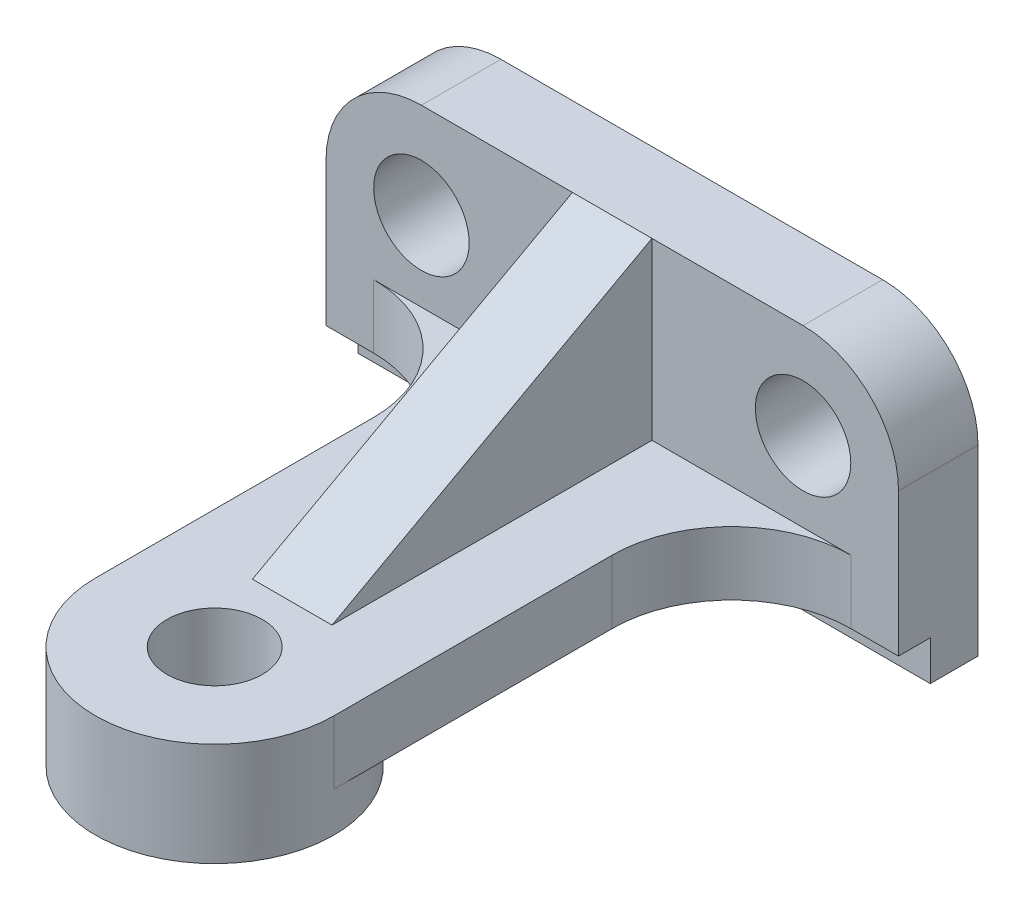
ISO-10303-21;
HEADER;
FILE_DESCRIPTION(('STEP AP214'),'2;1');
FILE_NAME('part.step','',(''),(''),'','','');
FILE_SCHEMA(('AUTOMOTIVE_DESIGN { 1 0 10303 214 1 1 1 1 }'));
ENDSEC;
DATA;
#1=APPLICATION_CONTEXT('core data for automotive mechanical design processes');
#2=APPLICATION_PROTOCOL_DEFINITION('international standard','automotive_design',2000,#1);
#3=PRODUCT_CONTEXT('',#1,'mechanical');
#4=PRODUCT('Part','Part','',(#3));
#5=PRODUCT_RELATED_PRODUCT_CATEGORY('part','',(#4));
#6=PRODUCT_DEFINITION_FORMATION('','',#4);
#7=PRODUCT_DEFINITION_CONTEXT('part definition',#1,'design');
#8=PRODUCT_DEFINITION('design','',#6,#7);
#9=PRODUCT_DEFINITION_SHAPE('','',#8);
#10=(LENGTH_UNIT() NAMED_UNIT(*) SI_UNIT(.MILLI.,.METRE.));
#11=(NAMED_UNIT(*) PLANE_ANGLE_UNIT() SI_UNIT($,.RADIAN.));
#12=(NAMED_UNIT(*) SI_UNIT($,.STERADIAN.) SOLID_ANGLE_UNIT());
#13=UNCERTAINTY_MEASURE_WITH_UNIT(LENGTH_MEASURE(1.E-05),#10,'distance_accuracy_value','');
#14=(GEOMETRIC_REPRESENTATION_CONTEXT(3) GLOBAL_UNCERTAINTY_ASSIGNED_CONTEXT((#13)) GLOBAL_UNIT_ASSIGNED_CONTEXT((#10,
#11,#12)) REPRESENTATION_CONTEXT('',''));
#15=CARTESIAN_POINT('',(0.,0.,0.));
#16=DIRECTION('',(0.,0.,1.));
#17=DIRECTION('',(1.,0.,0.));
#18=AXIS2_PLACEMENT_3D('',#15,#16,#17);
#19=CARTESIAN_POINT('',(42.,-9.99999999999999,50.2459304214752));
#20=DIRECTION('',(0.,0.877458255915555,0.479653009086393));
#21=DIRECTION('',(0.,-0.479653009086394,0.877458255915555));
#22=AXIS2_PLACEMENT_3D('',#19,#20,#21);
#23=PLANE('',#22);
#24=DIRECTION('',(0.,-0.479653009086393,0.877458255915555));
#25=VECTOR('',#24,1.);
#26=CARTESIAN_POINT('',(41.,12.,10.));
#27=LINE('',#26,#25);
#28=CARTESIAN_POINT('',(41.,12.,10.));
#29=VERTEX_POINT('',#28);
#30=CARTESIAN_POINT('',(41.,-9.99999999999999,50.2459304214752));
#31=VERTEX_POINT('',#30);
#32=EDGE_CURVE('E177',#29,#31,#27,.T.);
#33=ORIENTED_EDGE('',*,*,#32,.F.);
#34=DIRECTION('',(-1.,0.,0.));
#35=VECTOR('',#34,1.);
#36=CARTESIAN_POINT('',(42.,12.,10.));
#37=LINE('',#36,#35);
#38=CARTESIAN_POINT('',(31.,12.,10.));
#39=VERTEX_POINT('',#38);
#40=EDGE_CURVE('E186',#29,#39,#37,.T.);
#41=ORIENTED_EDGE('',*,*,#40,.T.);
#42=DIRECTION('',(0.,0.479653009086393,-0.877458255915555));
#43=VECTOR('',#42,1.);
#44=CARTESIAN_POINT('',(31.,-9.99999999999999,50.2459304214752));
#45=LINE('',#44,#43);
#46=CARTESIAN_POINT('',(31.,-9.99999999999999,50.2459304214752));
#47=VERTEX_POINT('',#46);
#48=EDGE_CURVE('E189',#47,#39,#45,.T.);
#49=ORIENTED_EDGE('',*,*,#48,.F.);
#50=DIRECTION('',(-1.,0.,0.));
#51=VECTOR('',#50,1.);
#52=CARTESIAN_POINT('',(42.,-9.99999999999999,50.2459304214752));
#53=LINE('',#52,#51);
#54=EDGE_CURVE('E171',#31,#47,#53,.T.);
#55=ORIENTED_EDGE('',*,*,#54,.F.);
#56=EDGE_LOOP('',(#33,#41,#49,#55));
#57=FACE_BOUND('',#56,.T.);
#58=ADVANCED_FACE('F44',(#57),#23,.T.);
#59=CARTESIAN_POINT('',(12.,0.,10.));
#60=DIRECTION('',(0.,0.,1.));
#61=DIRECTION('',(1.,0.,0.));
#62=AXIS2_PLACEMENT_3D('',#59,#60,#61);
#63=PLANE('',#62);
#64=CARTESIAN_POINT('',(60.,0.,10.));
#65=DIRECTION('',(0.,0.,1.));
#66=DIRECTION('',(1.,0.,0.));
#67=AXIS2_PLACEMENT_3D('',#64,#65,#66);
#68=CIRCLE('',#67,6.);
#69=CARTESIAN_POINT('',(66.,0.,10.));
#70=VERTEX_POINT('',#69);
#71=EDGE_CURVE('E205',#70,#70,#68,.T.);
#72=ORIENTED_EDGE('',*,*,#71,.F.);
#73=EDGE_LOOP('',(#72));
#74=FACE_BOUND('',#73,.T.);
#75=DIRECTION('',(-1.,0.,0.));
#76=VECTOR('',#75,1.);
#77=CARTESIAN_POINT('',(12.,12.,10.));
#78=LINE('',#77,#76);
#79=CARTESIAN_POINT('',(60.,12.,10.));
#80=VERTEX_POINT('',#79);
#81=EDGE_CURVE('E285',#80,#29,#78,.T.);
#82=ORIENTED_EDGE('',*,*,#81,.T.);
#83=DIRECTION('',(0.,1.,0.));
#84=VECTOR('',#83,1.);
#85=CARTESIAN_POINT('',(41.,-9.99999999999999,10.));
#86=LINE('',#85,#84);
#87=CARTESIAN_POINT('',(41.,-9.99999999999999,10.));
#88=VERTEX_POINT('',#87);
#89=EDGE_CURVE('E178',#88,#29,#86,.T.);
#90=ORIENTED_EDGE('',*,*,#89,.F.);
#91=DIRECTION('',(1.,0.,0.));
#92=VECTOR('',#91,1.);
#93=CARTESIAN_POINT('',(5.99999999999989,-9.99999999999999,10.));
#94=LINE('',#93,#92);
#95=CARTESIAN_POINT('',(66.0000000000001,-9.99999999999999,10.));
#96=VERTEX_POINT('',#95);
#97=EDGE_CURVE('E172',#88,#96,#94,.T.);
#98=ORIENTED_EDGE('',*,*,#97,.T.);
#99=DIRECTION('',(0.,-1.,0.));
#100=VECTOR('',#99,1.);
#101=CARTESIAN_POINT('',(66.0000000000001,-9.99999999999999,10.));
#102=LINE('',#101,#100);
#103=CARTESIAN_POINT('',(66.0000000000001,-18.,10.));
#104=VERTEX_POINT('',#103);
#105=EDGE_CURVE('E248',#96,#104,#102,.T.);
#106=ORIENTED_EDGE('',*,*,#105,.T.);
#107=DIRECTION('',(-1.,0.,0.));
#108=VECTOR('',#107,1.);
#109=CARTESIAN_POINT('',(72.,-18.,10.));
#110=LINE('',#109,#108);
#111=CARTESIAN_POINT('',(72.,-18.,10.));
#112=VERTEX_POINT('',#111);
#113=EDGE_CURVE('E271',#112,#104,#110,.T.);
#114=ORIENTED_EDGE('',*,*,#113,.F.);
#115=DIRECTION('',(0.,1.,0.));
#116=VECTOR('',#115,1.);
#117=CARTESIAN_POINT('',(72.,-23.,10.));
#118=LINE('',#117,#116);
#119=CARTESIAN_POINT('',(72.,0.,10.));
#120=VERTEX_POINT('',#119);
#121=EDGE_CURVE('E281',#112,#120,#118,.T.);
#122=ORIENTED_EDGE('',*,*,#121,.T.);
#123=CARTESIAN_POINT('',(60.,0.,10.));
#124=DIRECTION('',(0.,0.,1.));
#125=DIRECTION('',(1.,0.,0.));
#126=AXIS2_PLACEMENT_3D('',#123,#124,#125);
#127=CIRCLE('',#126,12.);
#128=EDGE_CURVE('E284',#120,#80,#127,.T.);
#129=ORIENTED_EDGE('',*,*,#128,.T.);
#130=EDGE_LOOP('',(#82,#90,#98,#106,#114,#122,#129));
#131=FACE_BOUND('',#130,.T.);
#132=ADVANCED_FACE('F332',(#74,#131),#63,.T.);
#133=CARTESIAN_POINT('',(72.,-18.,6.));
#134=DIRECTION('',(0.,1.,0.));
#135=DIRECTION('',(0.,0.,1.));
#136=AXIS2_PLACEMENT_3D('',#133,#134,#135);
#137=PLANE('',#136);
#138=CARTESIAN_POINT('',(36.,-18.,60.));
#139=DIRECTION('',(0.,-1.,0.));
#140=DIRECTION('',(0.,0.,-1.));
#141=AXIS2_PLACEMENT_3D('',#138,#139,#140);
#142=CIRCLE('',#141,15.);
#143=CARTESIAN_POINT('',(21.,-18.,60.));
#144=VERTEX_POINT('',#143);
#145=CARTESIAN_POINT('',(51.,-18.,60.));
#146=VERTEX_POINT('',#145);
#147=EDGE_CURVE('E206',#144,#146,#142,.T.);
#148=ORIENTED_EDGE('',*,*,#147,.F.);
#149=DIRECTION('',(0.,0.,-1.));
#150=VECTOR('',#149,1.);
#151=CARTESIAN_POINT('',(21.,-18.,60.));
#152=LINE('',#151,#150);
#153=CARTESIAN_POINT('',(21.,-18.,25.0000000000001));
#154=VERTEX_POINT('',#153);
#155=EDGE_CURVE('E217',#144,#154,#152,.T.);
#156=ORIENTED_EDGE('',*,*,#155,.T.);
#157=CARTESIAN_POINT('',(6.,-18.,25.));
#158=DIRECTION('',(0.,1.,0.));
#159=DIRECTION('',(0.,0.,1.));
#160=AXIS2_PLACEMENT_3D('',#157,#158,#159);
#161=CIRCLE('',#160,15.);
#162=CARTESIAN_POINT('',(6.,-18.,10.));
#163=VERTEX_POINT('',#162);
#164=EDGE_CURVE('E58',#154,#163,#161,.T.);
#165=ORIENTED_EDGE('',*,*,#164,.T.);
#166=CARTESIAN_POINT('',(0.,-18.,10.));
#167=VERTEX_POINT('',#166);
#168=EDGE_CURVE('E264',#163,#167,#110,.T.);
#169=ORIENTED_EDGE('',*,*,#168,.T.);
#170=DIRECTION('',(0.,0.,-1.));
#171=VECTOR('',#170,1.);
#172=CARTESIAN_POINT('',(0.,-18.,6.));
#173=LINE('',#172,#171);
#174=CARTESIAN_POINT('',(0.,-18.,6.));
#175=VERTEX_POINT('',#174);
#176=EDGE_CURVE('E246',#167,#175,#173,.T.);
#177=ORIENTED_EDGE('',*,*,#176,.T.);
#178=DIRECTION('',(-1.,0.,0.));
#179=VECTOR('',#178,1.);
#180=CARTESIAN_POINT('',(72.,-18.,6.));
#181=LINE('',#180,#179);
#182=CARTESIAN_POINT('',(72.,-18.,6.));
#183=VERTEX_POINT('',#182);
#184=EDGE_CURVE('E272',#183,#175,#181,.T.);
#185=ORIENTED_EDGE('',*,*,#184,.F.);
#186=DIRECTION('',(0.,0.,-1.));
#187=VECTOR('',#186,1.);
#188=CARTESIAN_POINT('',(72.,-18.,6.));
#189=LINE('',#188,#187);
#190=EDGE_CURVE('E67',#112,#183,#189,.T.);
#191=ORIENTED_EDGE('',*,*,#190,.F.);
#192=ORIENTED_EDGE('',*,*,#113,.T.);
#193=CARTESIAN_POINT('',(66.,-18.,25.));
#194=DIRECTION('',(0.,1.,0.));
#195=DIRECTION('',(0.,0.,-1.));
#196=AXIS2_PLACEMENT_3D('',#193,#194,#195);
#197=CIRCLE('',#196,15.);
#198=CARTESIAN_POINT('',(51.,-18.,25.0000000000001));
#199=VERTEX_POINT('',#198);
#200=EDGE_CURVE('E237',#104,#199,#197,.T.);
#201=ORIENTED_EDGE('',*,*,#200,.T.);
#202=DIRECTION('',(0.,0.,1.));
#203=VECTOR('',#202,1.);
#204=CARTESIAN_POINT('',(51.,-18.,60.));
#205=LINE('',#204,#203);
#206=EDGE_CURVE('E224',#199,#146,#205,.T.);
#207=ORIENTED_EDGE('',*,*,#206,.T.);
#208=EDGE_LOOP('',(#148,#156,#165,#169,#177,#185,#191,#192,#201,#207));
#209=FACE_BOUND('',#208,.T.);
#210=ADVANCED_FACE('F344',(#209),#137,.F.);
#211=CARTESIAN_POINT('',(12.,0.,10.));
#212=DIRECTION('',(0.,0.,-1.));
#213=DIRECTION('',(-1.,0.,0.));
#214=AXIS2_PLACEMENT_3D('',#211,#212,#213);
#215=CYLINDRICAL_SURFACE('',#214,12.);
#216=CARTESIAN_POINT('',(12.,0.,0.));
#217=DIRECTION('',(0.,0.,1.));
#218=DIRECTION('',(1.,0.,0.));
#219=AXIS2_PLACEMENT_3D('',#216,#217,#218);
#220=CIRCLE('',#219,12.);
#221=CARTESIAN_POINT('',(12.,12.,0.));
#222=VERTEX_POINT('',#221);
#223=CARTESIAN_POINT('',(0.,0.,0.));
#224=VERTEX_POINT('',#223);
#225=EDGE_CURVE('E267',#222,#224,#220,.T.);
#226=ORIENTED_EDGE('',*,*,#225,.T.);
#227=DIRECTION('',(0.,0.,-1.));
#228=VECTOR('',#227,1.);
#229=CARTESIAN_POINT('',(0.,0.,10.));
#230=LINE('',#229,#228);
#231=CARTESIAN_POINT('',(0.,0.,10.));
#232=VERTEX_POINT('',#231);
#233=EDGE_CURVE('E11',#232,#224,#230,.T.);
#234=ORIENTED_EDGE('',*,*,#233,.F.);
#235=CARTESIAN_POINT('',(12.,0.,10.));
#236=DIRECTION('',(0.,0.,1.));
#237=DIRECTION('',(1.,0.,0.));
#238=AXIS2_PLACEMENT_3D('',#235,#236,#237);
#239=CIRCLE('',#238,12.);
#240=CARTESIAN_POINT('',(12.,12.,10.));
#241=VERTEX_POINT('',#240);
#242=EDGE_CURVE('E273',#241,#232,#239,.T.);
#243=ORIENTED_EDGE('',*,*,#242,.F.);
#244=DIRECTION('',(0.,0.,-1.));
#245=VECTOR('',#244,1.);
#246=CARTESIAN_POINT('',(12.,12.,10.));
#247=LINE('',#246,#245);
#248=EDGE_CURVE('E290',#241,#222,#247,.T.);
#249=ORIENTED_EDGE('',*,*,#248,.T.);
#250=EDGE_LOOP('',(#226,#234,#243,#249));
#251=FACE_BOUND('',#250,.T.);
#252=ADVANCED_FACE('F50',(#251),#215,.T.);
#253=CARTESIAN_POINT('',(0.,0.,10.));
#254=DIRECTION('',(1.,0.,0.));
#255=DIRECTION('',(0.,0.,-1.));
#256=AXIS2_PLACEMENT_3D('',#253,#254,#255);
#257=PLANE('',#256);
#258=DIRECTION('',(0.,-1.,0.));
#259=VECTOR('',#258,1.);
#260=CARTESIAN_POINT('',(0.,0.,10.));
#261=LINE('',#260,#259);
#262=EDGE_CURVE('E280',#232,#167,#261,.T.);
#263=ORIENTED_EDGE('',*,*,#262,.F.);
#264=ORIENTED_EDGE('',*,*,#233,.T.);
#265=DIRECTION('',(0.,-1.,0.));
#266=VECTOR('',#265,1.);
#267=CARTESIAN_POINT('',(0.,0.,0.));
#268=LINE('',#267,#266);
#269=CARTESIAN_POINT('',(0.,-23.,0.));
#270=VERTEX_POINT('',#269);
#271=EDGE_CURVE('E287',#224,#270,#268,.T.);
#272=ORIENTED_EDGE('',*,*,#271,.T.);
#273=DIRECTION('',(0.,0.,-1.));
#274=VECTOR('',#273,1.);
#275=CARTESIAN_POINT('',(0.,-23.,10.));
#276=LINE('',#275,#274);
#277=CARTESIAN_POINT('',(0.,-23.,6.));
#278=VERTEX_POINT('',#277);
#279=EDGE_CURVE('E52',#278,#270,#276,.T.);
#280=ORIENTED_EDGE('',*,*,#279,.F.);
#281=DIRECTION('',(0.,-1.,0.));
#282=VECTOR('',#281,1.);
#283=CARTESIAN_POINT('',(0.,-23.,6.));
#284=LINE('',#283,#282);
#285=EDGE_CURVE('E257',#175,#278,#284,.T.);
#286=ORIENTED_EDGE('',*,*,#285,.F.);
#287=ORIENTED_EDGE('',*,*,#176,.F.);
#288=EDGE_LOOP('',(#263,#264,#272,#280,#286,#287));
#289=FACE_BOUND('',#288,.T.);
#290=ADVANCED_FACE('F319',(#289),#257,.F.);
#291=CARTESIAN_POINT('',(0.,-23.,10.));
#292=DIRECTION('',(0.,1.,0.));
#293=DIRECTION('',(0.,0.,1.));
#294=AXIS2_PLACEMENT_3D('',#291,#292,#293);
#295=PLANE('',#294);
#296=DIRECTION('',(0.,0.,-1.));
#297=VECTOR('',#296,1.);
#298=CARTESIAN_POINT('',(72.,-23.,10.));
#299=LINE('',#298,#297);
#300=CARTESIAN_POINT('',(72.,-23.,6.));
#301=VERTEX_POINT('',#300);
#302=CARTESIAN_POINT('',(72.,-23.,0.));
#303=VERTEX_POINT('',#302);
#304=EDGE_CURVE('E307',#301,#303,#299,.T.);
#305=ORIENTED_EDGE('',*,*,#304,.F.);
#306=DIRECTION('',(-1.,0.,0.));
#307=VECTOR('',#306,1.);
#308=CARTESIAN_POINT('',(72.,-23.,6.));
#309=LINE('',#308,#307);
#310=EDGE_CURVE('E270',#301,#278,#309,.T.);
#311=ORIENTED_EDGE('',*,*,#310,.T.);
#312=ORIENTED_EDGE('',*,*,#279,.T.);
#313=DIRECTION('',(1.,0.,0.));
#314=VECTOR('',#313,1.);
#315=CARTESIAN_POINT('',(0.,-23.,0.));
#316=LINE('',#315,#314);
#317=EDGE_CURVE('E291',#270,#303,#316,.T.);
#318=ORIENTED_EDGE('',*,*,#317,.T.);
#319=EDGE_LOOP('',(#305,#311,#312,#318));
#320=FACE_BOUND('',#319,.T.);
#321=ADVANCED_FACE('F312',(#320),#295,.F.);
#322=CARTESIAN_POINT('',(72.,-23.,10.));
#323=DIRECTION('',(-1.,0.,0.));
#324=DIRECTION('',(0.,0.,1.));
#325=AXIS2_PLACEMENT_3D('',#322,#323,#324);
#326=PLANE('',#325);
#327=ORIENTED_EDGE('',*,*,#190,.T.);
#328=DIRECTION('',(0.,-1.,0.));
#329=VECTOR('',#328,1.);
#330=CARTESIAN_POINT('',(72.,-23.,6.));
#331=LINE('',#330,#329);
#332=EDGE_CURVE('E258',#183,#301,#331,.T.);
#333=ORIENTED_EDGE('',*,*,#332,.T.);
#334=ORIENTED_EDGE('',*,*,#304,.T.);
#335=DIRECTION('',(0.,1.,0.));
#336=VECTOR('',#335,1.);
#337=CARTESIAN_POINT('',(72.,-23.,0.));
#338=LINE('',#337,#336);
#339=CARTESIAN_POINT('',(72.,0.,0.));
#340=VERTEX_POINT('',#339);
#341=EDGE_CURVE('E298',#303,#340,#338,.T.);
#342=ORIENTED_EDGE('',*,*,#341,.T.);
#343=DIRECTION('',(0.,0.,-1.));
#344=VECTOR('',#343,1.);
#345=CARTESIAN_POINT('',(72.,0.,10.));
#346=LINE('',#345,#344);
#347=EDGE_CURVE('E306',#120,#340,#346,.T.);
#348=ORIENTED_EDGE('',*,*,#347,.F.);
#349=ORIENTED_EDGE('',*,*,#121,.F.);
#350=EDGE_LOOP('',(#327,#333,#334,#342,#348,#349));
#351=FACE_BOUND('',#350,.T.);
#352=ADVANCED_FACE('F327',(#351),#326,.F.);
#353=CARTESIAN_POINT('',(60.,0.,10.));
#354=DIRECTION('',(0.,0.,-1.));
#355=DIRECTION('',(-1.,0.,0.));
#356=AXIS2_PLACEMENT_3D('',#353,#354,#355);
#357=CYLINDRICAL_SURFACE('',#356,12.);
#358=CARTESIAN_POINT('',(60.,0.,0.));
#359=DIRECTION('',(0.,0.,1.));
#360=DIRECTION('',(1.,0.,0.));
#361=AXIS2_PLACEMENT_3D('',#358,#359,#360);
#362=CIRCLE('',#361,12.);
#363=CARTESIAN_POINT('',(60.,12.,0.));
#364=VERTEX_POINT('',#363);
#365=EDGE_CURVE('E296',#340,#364,#362,.T.);
#366=ORIENTED_EDGE('',*,*,#365,.T.);
#367=DIRECTION('',(0.,0.,-1.));
#368=VECTOR('',#367,1.);
#369=CARTESIAN_POINT('',(60.,12.,10.));
#370=LINE('',#369,#368);
#371=EDGE_CURVE('E303',#80,#364,#370,.T.);
#372=ORIENTED_EDGE('',*,*,#371,.F.);
#373=ORIENTED_EDGE('',*,*,#128,.F.);
#374=ORIENTED_EDGE('',*,*,#347,.T.);
#375=EDGE_LOOP('',(#366,#372,#373,#374));
#376=FACE_BOUND('',#375,.T.);
#377=ADVANCED_FACE('F333',(#376),#357,.T.);
#378=CARTESIAN_POINT('',(12.,12.,10.));
#379=DIRECTION('',(0.,-1.,0.));
#380=DIRECTION('',(1.,0.,0.));
#381=AXIS2_PLACEMENT_3D('',#378,#379,#380);
#382=PLANE('',#381);
#383=DIRECTION('',(-1.,0.,0.));
#384=VECTOR('',#383,1.);
#385=CARTESIAN_POINT('',(12.,12.,0.));
#386=LINE('',#385,#384);
#387=EDGE_CURVE('E278',#364,#222,#386,.T.);
#388=ORIENTED_EDGE('',*,*,#387,.T.);
#389=ORIENTED_EDGE('',*,*,#248,.F.);
#390=DIRECTION('',(-1.,0.,0.));
#391=VECTOR('',#390,1.);
#392=CARTESIAN_POINT('',(30.,12.,10.));
#393=LINE('',#392,#391);
#394=EDGE_CURVE('E350',#39,#241,#393,.T.);
#395=ORIENTED_EDGE('',*,*,#394,.F.);
#396=ORIENTED_EDGE('',*,*,#40,.F.);
#397=ORIENTED_EDGE('',*,*,#81,.F.);
#398=ORIENTED_EDGE('',*,*,#371,.T.);
#399=EDGE_LOOP('',(#388,#389,#395,#396,#397,#398));
#400=FACE_BOUND('',#399,.T.);
#401=ADVANCED_FACE('F354',(#400),#382,.F.);
#402=DIRECTION('',(0.,-1.,0.));
#403=VECTOR('',#402,1.);
#404=CARTESIAN_POINT('',(5.9999999999999,-9.99999999999999,10.));
#405=LINE('',#404,#403);
#406=CARTESIAN_POINT('',(5.9999999999999,-9.99999999999999,10.));
#407=VERTEX_POINT('',#406);
#408=EDGE_CURVE('E255',#407,#163,#405,.T.);
#409=ORIENTED_EDGE('',*,*,#408,.F.);
#410=DIRECTION('',(-1.,0.,0.));
#411=VECTOR('',#410,1.);
#412=CARTESIAN_POINT('',(30.,-9.99999999999999,10.));
#413=LINE('',#412,#411);
#414=CARTESIAN_POINT('',(31.,-9.99999999999999,10.));
#415=VERTEX_POINT('',#414);
#416=EDGE_CURVE('E192',#415,#407,#413,.T.);
#417=ORIENTED_EDGE('',*,*,#416,.F.);
#418=DIRECTION('',(0.,-1.,0.));
#419=VECTOR('',#418,1.);
#420=CARTESIAN_POINT('',(31.,12.,10.));
#421=LINE('',#420,#419);
#422=EDGE_CURVE('E357',#39,#415,#421,.T.);
#423=ORIENTED_EDGE('',*,*,#422,.F.);
#424=ORIENTED_EDGE('',*,*,#394,.T.);
#425=ORIENTED_EDGE('',*,*,#242,.T.);
#426=ORIENTED_EDGE('',*,*,#262,.T.);
#427=ORIENTED_EDGE('',*,*,#168,.F.);
#428=EDGE_LOOP('',(#409,#417,#423,#424,#425,#426,#427));
#429=FACE_BOUND('',#428,.T.);
#430=CARTESIAN_POINT('',(12.,0.,10.));
#431=DIRECTION('',(0.,0.,-1.));
#432=DIRECTION('',(0.,1.,0.));
#433=AXIS2_PLACEMENT_3D('',#430,#431,#432);
#434=CIRCLE('',#433,6.);
#435=CARTESIAN_POINT('',(12.,6.,10.));
#436=VERTEX_POINT('',#435);
#437=EDGE_CURVE('E188',#436,#436,#434,.F.);
#438=ORIENTED_EDGE('',*,*,#437,.F.);
#439=EDGE_LOOP('',(#438));
#440=FACE_BOUND('',#439,.T.);
#441=ADVANCED_FACE('F342',(#429,#440),#63,.T.);
#442=CARTESIAN_POINT('',(12.,0.,0.));
#443=DIRECTION('',(0.,0.,1.));
#444=DIRECTION('',(1.,0.,0.));
#445=AXIS2_PLACEMENT_3D('',#442,#443,#444);
#446=PLANE('',#445);
#447=CARTESIAN_POINT('',(12.,0.,0.));
#448=DIRECTION('',(0.,0.,1.));
#449=DIRECTION('',(1.,0.,0.));
#450=AXIS2_PLACEMENT_3D('',#447,#448,#449);
#451=CIRCLE('',#450,6.);
#452=CARTESIAN_POINT('',(18.,0.,0.));
#453=VERTEX_POINT('',#452);
#454=EDGE_CURVE('E202',#453,#453,#451,.T.);
#455=ORIENTED_EDGE('',*,*,#454,.T.);
#456=EDGE_LOOP('',(#455));
#457=FACE_BOUND('',#456,.T.);
#458=CARTESIAN_POINT('',(60.,0.,0.));
#459=DIRECTION('',(0.,0.,1.));
#460=DIRECTION('',(1.,0.,0.));
#461=AXIS2_PLACEMENT_3D('',#458,#459,#460);
#462=CIRCLE('',#461,6.);
#463=CARTESIAN_POINT('',(66.,0.,0.));
#464=VERTEX_POINT('',#463);
#465=EDGE_CURVE('E209',#464,#464,#462,.T.);
#466=ORIENTED_EDGE('',*,*,#465,.T.);
#467=EDGE_LOOP('',(#466));
#468=FACE_BOUND('',#467,.T.);
#469=ORIENTED_EDGE('',*,*,#225,.F.);
#470=ORIENTED_EDGE('',*,*,#387,.F.);
#471=ORIENTED_EDGE('',*,*,#365,.F.);
#472=ORIENTED_EDGE('',*,*,#341,.F.);
#473=ORIENTED_EDGE('',*,*,#317,.F.);
#474=ORIENTED_EDGE('',*,*,#271,.F.);
#475=EDGE_LOOP('',(#469,#470,#471,#472,#473,#474));
#476=FACE_BOUND('',#475,.T.);
#477=ADVANCED_FACE('F321',(#457,#468,#476),#446,.F.);
#478=CARTESIAN_POINT('',(72.,-23.,6.));
#479=DIRECTION('',(0.,0.,-1.));
#480=DIRECTION('',(-1.,0.,0.));
#481=AXIS2_PLACEMENT_3D('',#478,#479,#480);
#482=PLANE('',#481);
#483=ORIENTED_EDGE('',*,*,#285,.T.);
#484=ORIENTED_EDGE('',*,*,#310,.F.);
#485=ORIENTED_EDGE('',*,*,#332,.F.);
#486=ORIENTED_EDGE('',*,*,#184,.T.);
#487=EDGE_LOOP('',(#483,#484,#485,#486));
#488=FACE_BOUND('',#487,.T.);
#489=ADVANCED_FACE('F336',(#488),#482,.F.);
#490=CARTESIAN_POINT('',(36.,-9.99999999999999,60.));
#491=DIRECTION('',(0.,-1.,0.));
#492=DIRECTION('',(0.,0.,-1.));
#493=AXIS2_PLACEMENT_3D('',#490,#491,#492);
#494=CYLINDRICAL_SURFACE('',#493,15.);
#495=DIRECTION('',(0.,-1.,0.));
#496=VECTOR('',#495,1.);
#497=CARTESIAN_POINT('',(21.,-9.99999999999999,60.));
#498=LINE('',#497,#496);
#499=CARTESIAN_POINT('',(21.,-9.99999999999999,60.));
#500=VERTEX_POINT('',#499);
#501=EDGE_CURVE('E236',#500,#144,#498,.T.);
#502=ORIENTED_EDGE('',*,*,#501,.T.);
#503=ORIENTED_EDGE('',*,*,#147,.T.);
#504=DIRECTION('',(0.,-1.,0.));
#505=VECTOR('',#504,1.);
#506=CARTESIAN_POINT('',(51.,-9.99999999999999,60.));
#507=LINE('',#506,#505);
#508=CARTESIAN_POINT('',(51.,-9.99999999999999,60.));
#509=VERTEX_POINT('',#508);
#510=EDGE_CURVE('E242',#509,#146,#507,.T.);
#511=ORIENTED_EDGE('',*,*,#510,.F.);
#512=CARTESIAN_POINT('',(36.,-9.99999999999999,60.));
#513=DIRECTION('',(0.,-1.,0.));
#514=DIRECTION('',(0.,0.,-1.));
#515=AXIS2_PLACEMENT_3D('',#512,#513,#514);
#516=CIRCLE('',#515,15.);
#517=EDGE_CURVE('E220',#509,#500,#516,.T.);
#518=ORIENTED_EDGE('',*,*,#517,.T.);
#519=EDGE_LOOP('',(#502,#503,#511,#518));
#520=FACE_BOUND('',#519,.T.);
#521=CARTESIAN_POINT('',(36.,-23.,60.));
#522=DIRECTION('',(0.,-1.,0.));
#523=DIRECTION('',(0.,0.,-1.));
#524=AXIS2_PLACEMENT_3D('',#521,#522,#523);
#525=CIRCLE('',#524,15.);
#526=CARTESIAN_POINT('',(36.,-23.,45.));
#527=VERTEX_POINT('',#526);
#528=EDGE_CURVE('E213',#527,#527,#525,.T.);
#529=ORIENTED_EDGE('',*,*,#528,.F.);
#530=EDGE_LOOP('',(#529));
#531=FACE_BOUND('',#530,.T.);
#532=ADVANCED_FACE('F374',(#520,#531),#494,.T.);
#533=CARTESIAN_POINT('',(51.,-9.99999999999999,60.));
#534=DIRECTION('',(1.,0.,0.));
#535=DIRECTION('',(0.,0.,-1.));
#536=AXIS2_PLACEMENT_3D('',#533,#534,#535);
#537=PLANE('',#536);
#538=ORIENTED_EDGE('',*,*,#206,.F.);
#539=DIRECTION('',(0.,-1.,0.));
#540=VECTOR('',#539,1.);
#541=CARTESIAN_POINT('',(51.,-9.99999999999999,25.0000000000001));
#542=LINE('',#541,#540);
#543=CARTESIAN_POINT('',(51.,-9.99999999999999,25.0000000000001));
#544=VERTEX_POINT('',#543);
#545=EDGE_CURVE('E250',#544,#199,#542,.T.);
#546=ORIENTED_EDGE('',*,*,#545,.F.);
#547=DIRECTION('',(0.,0.,1.));
#548=VECTOR('',#547,1.);
#549=CARTESIAN_POINT('',(51.,-9.99999999999999,60.));
#550=LINE('',#549,#548);
#551=EDGE_CURVE('E231',#544,#509,#550,.T.);
#552=ORIENTED_EDGE('',*,*,#551,.T.);
#553=ORIENTED_EDGE('',*,*,#510,.T.);
#554=EDGE_LOOP('',(#538,#546,#552,#553));
#555=FACE_BOUND('',#554,.T.);
#556=ADVANCED_FACE('F378',(#555),#537,.T.);
#557=CARTESIAN_POINT('',(66.,-9.99999999999999,25.));
#558=DIRECTION('',(0.,-1.,0.));
#559=DIRECTION('',(0.,0.,-1.));
#560=AXIS2_PLACEMENT_3D('',#557,#558,#559);
#561=CYLINDRICAL_SURFACE('',#560,15.);
#562=ORIENTED_EDGE('',*,*,#200,.F.);
#563=ORIENTED_EDGE('',*,*,#105,.F.);
#564=CARTESIAN_POINT('',(66.,-9.99999999999999,25.));
#565=DIRECTION('',(0.,1.,0.));
#566=DIRECTION('',(0.,0.,-1.));
#567=AXIS2_PLACEMENT_3D('',#564,#565,#566);
#568=CIRCLE('',#567,15.);
#569=EDGE_CURVE('E229',#96,#544,#568,.T.);
#570=ORIENTED_EDGE('',*,*,#569,.T.);
#571=ORIENTED_EDGE('',*,*,#545,.T.);
#572=EDGE_LOOP('',(#562,#563,#570,#571));
#573=FACE_BOUND('',#572,.T.);
#574=ADVANCED_FACE('F385',(#573),#561,.F.);
#575=CARTESIAN_POINT('',(6.,-9.99999999999999,25.));
#576=DIRECTION('',(0.,-1.,0.));
#577=DIRECTION('',(0.,0.,-1.));
#578=AXIS2_PLACEMENT_3D('',#575,#576,#577);
#579=CYLINDRICAL_SURFACE('',#578,15.);
#580=ORIENTED_EDGE('',*,*,#164,.F.);
#581=DIRECTION('',(0.,-1.,0.));
#582=VECTOR('',#581,1.);
#583=CARTESIAN_POINT('',(21.,-9.99999999999999,25.0000000000001));
#584=LINE('',#583,#582);
#585=CARTESIAN_POINT('',(21.,-9.99999999999999,25.0000000000001));
#586=VERTEX_POINT('',#585);
#587=EDGE_CURVE('E251',#586,#154,#584,.T.);
#588=ORIENTED_EDGE('',*,*,#587,.F.);
#589=CARTESIAN_POINT('',(6.,-9.99999999999999,25.));
#590=DIRECTION('',(0.,1.,0.));
#591=DIRECTION('',(0.,0.,1.));
#592=AXIS2_PLACEMENT_3D('',#589,#590,#591);
#593=CIRCLE('',#592,15.);
#594=EDGE_CURVE('E228',#586,#407,#593,.T.);
#595=ORIENTED_EDGE('',*,*,#594,.T.);
#596=ORIENTED_EDGE('',*,*,#408,.T.);
#597=EDGE_LOOP('',(#580,#588,#595,#596));
#598=FACE_BOUND('',#597,.T.);
#599=ADVANCED_FACE('F367',(#598),#579,.F.);
#600=CARTESIAN_POINT('',(21.,-9.99999999999999,60.));
#601=DIRECTION('',(-1.,0.,0.));
#602=DIRECTION('',(0.,0.,1.));
#603=AXIS2_PLACEMENT_3D('',#600,#601,#602);
#604=PLANE('',#603);
#605=ORIENTED_EDGE('',*,*,#155,.F.);
#606=ORIENTED_EDGE('',*,*,#501,.F.);
#607=DIRECTION('',(0.,0.,-1.));
#608=VECTOR('',#607,1.);
#609=CARTESIAN_POINT('',(21.,-9.99999999999999,60.));
#610=LINE('',#609,#608);
#611=EDGE_CURVE('E221',#500,#586,#610,.T.);
#612=ORIENTED_EDGE('',*,*,#611,.T.);
#613=ORIENTED_EDGE('',*,*,#587,.T.);
#614=EDGE_LOOP('',(#605,#606,#612,#613));
#615=FACE_BOUND('',#614,.T.);
#616=ADVANCED_FACE('F371',(#615),#604,.T.);
#617=CARTESIAN_POINT('',(36.,-9.99999999999999,60.));
#618=DIRECTION('',(0.,-1.,0.));
#619=DIRECTION('',(0.,0.,-1.));
#620=AXIS2_PLACEMENT_3D('',#617,#618,#619);
#621=PLANE('',#620);
#622=DIRECTION('',(0.,0.,-1.));
#623=VECTOR('',#622,1.);
#624=CARTESIAN_POINT('',(41.,-9.99999999999999,50.2459304214752));
#625=LINE('',#624,#623);
#626=EDGE_CURVE('E164',#31,#88,#625,.T.);
#627=ORIENTED_EDGE('',*,*,#626,.F.);
#628=ORIENTED_EDGE('',*,*,#54,.T.);
#629=DIRECTION('',(0.,0.,1.));
#630=VECTOR('',#629,1.);
#631=CARTESIAN_POINT('',(31.,-9.99999999999999,10.));
#632=LINE('',#631,#630);
#633=EDGE_CURVE('E352',#415,#47,#632,.T.);
#634=ORIENTED_EDGE('',*,*,#633,.F.);
#635=ORIENTED_EDGE('',*,*,#416,.T.);
#636=ORIENTED_EDGE('',*,*,#594,.F.);
#637=ORIENTED_EDGE('',*,*,#611,.F.);
#638=ORIENTED_EDGE('',*,*,#517,.F.);
#639=ORIENTED_EDGE('',*,*,#551,.F.);
#640=ORIENTED_EDGE('',*,*,#569,.F.);
#641=ORIENTED_EDGE('',*,*,#97,.F.);
#642=EDGE_LOOP('',(#627,#628,#634,#635,#636,#637,#638,#639,#640,#641));
#643=FACE_BOUND('',#642,.T.);
#644=CARTESIAN_POINT('',(36.,-10.,60.));
#645=DIRECTION('',(0.,-1.,0.));
#646=DIRECTION('',(0.,0.,-1.));
#647=AXIS2_PLACEMENT_3D('',#644,#645,#646);
#648=CIRCLE('',#647,5.99999999999999);
#649=CARTESIAN_POINT('',(36.,-9.99999999999999,54.));
#650=VERTEX_POINT('',#649);
#651=EDGE_CURVE('E198',#650,#650,#648,.T.);
#652=ORIENTED_EDGE('',*,*,#651,.T.);
#653=EDGE_LOOP('',(#652));
#654=FACE_BOUND('',#653,.T.);
#655=ADVANCED_FACE('F170',(#643,#654),#621,.F.);
#656=CARTESIAN_POINT('',(36.,-23.,60.));
#657=DIRECTION('',(0.,-1.,0.));
#658=DIRECTION('',(0.,0.,-1.));
#659=AXIS2_PLACEMENT_3D('',#656,#657,#658);
#660=PLANE('',#659);
#661=CARTESIAN_POINT('',(36.,-23.,60.));
#662=DIRECTION('',(0.,-1.,0.));
#663=DIRECTION('',(0.,0.,-1.));
#664=AXIS2_PLACEMENT_3D('',#661,#662,#663);
#665=CIRCLE('',#664,5.99999999999999);
#666=CARTESIAN_POINT('',(36.,-23.,54.));
#667=VERTEX_POINT('',#666);
#668=EDGE_CURVE('E191',#667,#667,#665,.T.);
#669=ORIENTED_EDGE('',*,*,#668,.F.);
#670=EDGE_LOOP('',(#669));
#671=FACE_BOUND('',#670,.T.);
#672=ORIENTED_EDGE('',*,*,#528,.T.);
#673=EDGE_LOOP('',(#672));
#674=FACE_BOUND('',#673,.T.);
#675=ADVANCED_FACE('F414',(#671,#674),#660,.T.);
#676=CARTESIAN_POINT('',(60.,0.,0.));
#677=DIRECTION('',(0.,0.,1.));
#678=DIRECTION('',(1.,0.,0.));
#679=AXIS2_PLACEMENT_3D('',#676,#677,#678);
#680=CYLINDRICAL_SURFACE('',#679,6.);
#681=ORIENTED_EDGE('',*,*,#465,.F.);
#682=EDGE_LOOP('',(#681));
#683=FACE_BOUND('',#682,.T.);
#684=ORIENTED_EDGE('',*,*,#71,.T.);
#685=EDGE_LOOP('',(#684));
#686=FACE_BOUND('',#685,.T.);
#687=ADVANCED_FACE('F408',(#683,#686),#680,.F.);
#688=CARTESIAN_POINT('',(12.,0.,0.));
#689=DIRECTION('',(0.,0.,1.));
#690=DIRECTION('',(1.,0.,0.));
#691=AXIS2_PLACEMENT_3D('',#688,#689,#690);
#692=CYLINDRICAL_SURFACE('',#691,6.);
#693=ORIENTED_EDGE('',*,*,#454,.F.);
#694=EDGE_LOOP('',(#693));
#695=FACE_BOUND('',#694,.T.);
#696=ORIENTED_EDGE('',*,*,#437,.T.);
#697=EDGE_LOOP('',(#696));
#698=FACE_BOUND('',#697,.T.);
#699=ADVANCED_FACE('F403',(#695,#698),#692,.F.);
#700=CARTESIAN_POINT('',(36.,-10.,60.));
#701=DIRECTION('',(0.,-1.,0.));
#702=DIRECTION('',(0.,0.,-1.));
#703=AXIS2_PLACEMENT_3D('',#700,#701,#702);
#704=CYLINDRICAL_SURFACE('',#703,5.99999999999999);
#705=CARTESIAN_POINT('',(36.,-9.99999999999999,54.));
#706=CARTESIAN_POINT('',(36.,-10.1354166666667,54.));
#707=CARTESIAN_POINT('',(36.,-10.2708333333333,54.));
#708=CARTESIAN_POINT('',(36.,-10.5416666666667,54.));
#709=CARTESIAN_POINT('',(36.,-10.6770833333333,54.));
#710=CARTESIAN_POINT('',(36.,-10.9479166666667,54.));
#711=CARTESIAN_POINT('',(36.,-11.0833333333333,54.));
#712=CARTESIAN_POINT('',(36.,-11.3541666666667,54.));
#713=CARTESIAN_POINT('',(36.,-11.4895833333333,54.));
#714=CARTESIAN_POINT('',(36.,-11.7604166666667,54.));
#715=CARTESIAN_POINT('',(36.,-11.8958333333333,54.));
#716=CARTESIAN_POINT('',(36.,-12.1666666666667,54.));
#717=CARTESIAN_POINT('',(36.,-12.3020833333333,54.));
#718=CARTESIAN_POINT('',(36.,-12.5729166666667,54.));
#719=CARTESIAN_POINT('',(36.,-12.7083333333333,54.));
#720=CARTESIAN_POINT('',(36.,-12.9791666666667,54.));
#721=CARTESIAN_POINT('',(36.,-13.1145833333333,54.));
#722=CARTESIAN_POINT('',(36.,-13.3854166666667,54.));
#723=CARTESIAN_POINT('',(36.,-13.5208333333333,54.));
#724=CARTESIAN_POINT('',(36.,-13.7916666666667,54.));
#725=CARTESIAN_POINT('',(36.,-13.9270833333333,54.));
#726=CARTESIAN_POINT('',(36.,-14.1979166666667,54.));
#727=CARTESIAN_POINT('',(36.,-14.3333333333333,54.));
#728=CARTESIAN_POINT('',(36.,-14.6041666666667,54.));
#729=CARTESIAN_POINT('',(36.,-14.7395833333333,54.));
#730=CARTESIAN_POINT('',(36.,-15.0104166666667,54.));
#731=CARTESIAN_POINT('',(36.,-15.1458333333333,54.));
#732=CARTESIAN_POINT('',(36.,-15.4166666666667,54.));
#733=CARTESIAN_POINT('',(36.,-15.5520833333333,54.));
#734=CARTESIAN_POINT('',(36.,-15.8229166666667,54.));
#735=CARTESIAN_POINT('',(36.,-15.9583333333333,54.));
#736=CARTESIAN_POINT('',(36.,-16.2291666666667,54.));
#737=CARTESIAN_POINT('',(36.,-16.3645833333333,54.));
#738=CARTESIAN_POINT('',(36.,-16.6354166666667,54.));
#739=CARTESIAN_POINT('',(36.,-16.7708333333333,54.));
#740=CARTESIAN_POINT('',(36.,-17.0416666666667,54.));
#741=CARTESIAN_POINT('',(36.,-17.1770833333333,54.));
#742=CARTESIAN_POINT('',(36.,-17.4479166666667,54.));
#743=CARTESIAN_POINT('',(36.,-17.5833333333333,54.));
#744=CARTESIAN_POINT('',(36.,-17.8541666666667,54.));
#745=CARTESIAN_POINT('',(36.,-17.9895833333333,54.));
#746=CARTESIAN_POINT('',(36.,-18.2604166666667,54.));
#747=CARTESIAN_POINT('',(36.,-18.3958333333333,54.));
#748=CARTESIAN_POINT('',(36.,-18.6666666666667,54.));
#749=CARTESIAN_POINT('',(36.,-18.8020833333333,54.));
#750=CARTESIAN_POINT('',(36.,-19.0729166666667,54.));
#751=CARTESIAN_POINT('',(36.,-19.2083333333333,54.));
#752=CARTESIAN_POINT('',(36.,-19.4791666666667,54.));
#753=CARTESIAN_POINT('',(36.,-19.6145833333333,54.));
#754=CARTESIAN_POINT('',(36.,-19.8854166666667,54.));
#755=CARTESIAN_POINT('',(36.,-20.0208333333333,54.));
#756=CARTESIAN_POINT('',(36.,-20.2916666666667,54.));
#757=CARTESIAN_POINT('',(36.,-20.4270833333333,54.));
#758=CARTESIAN_POINT('',(36.,-20.6979166666667,54.));
#759=CARTESIAN_POINT('',(36.,-20.8333333333333,54.));
#760=CARTESIAN_POINT('',(36.,-21.1041666666667,54.));
#761=CARTESIAN_POINT('',(36.,-21.2395833333333,54.));
#762=CARTESIAN_POINT('',(36.,-21.5104166666667,54.));
#763=CARTESIAN_POINT('',(36.,-21.6458333333333,54.));
#764=CARTESIAN_POINT('',(36.,-21.9166666666667,54.));
#765=CARTESIAN_POINT('',(36.,-22.0520833333333,54.));
#766=CARTESIAN_POINT('',(36.,-22.3229166666667,54.));
#767=CARTESIAN_POINT('',(36.,-22.4583333333333,54.));
#768=CARTESIAN_POINT('',(36.,-22.7291666666667,54.));
#769=CARTESIAN_POINT('',(36.,-22.8645833333333,54.));
#770=CARTESIAN_POINT('',(36.,-23.,54.));
#771=B_SPLINE_CURVE_WITH_KNOTS('',3,(#705,#706,#707,#708,#709,#710,#711,#712,#713,#714,#715,
#716,#717,#718,#719,#720,#721,#722,#723,#724,#725,#726,#727,#728,#729,#730,#731,#732,#733,#734,
#735,#736,#737,#738,#739,#740,#741,#742,#743,#744,#745,#746,#747,#748,#749,#750,#751,#752,#753,
#754,#755,#756,#757,#758,#759,#760,#761,#762,#763,#764,#765,#766,#767,#768,#769,#770),
.UNSPECIFIED.,.F.,.F.,(4,2,2,2,2,2,2,2,2,2,2,2,2,2,2,2,2,2,2,2,2,2,2,2,2,2,2,2,2,2,2,2,4),(0.,
0.40625,0.812500000000001,1.21875,1.625,2.03125,2.4375,2.84375,3.25,3.65625,4.0625,4.46875,
4.875,5.28125,5.6875,6.09375,6.5,6.90625,7.3125,7.71875,8.125,8.53125,8.9375,9.34375,9.75,
10.15625,10.5625,10.96875,11.375,11.78125,12.1875,12.59375,13.),.UNSPECIFIED.);
#772=EDGE_CURVE('BSEAM405',#650,#667,#771,.T.);
#773=ORIENTED_EDGE('',*,*,#651,.F.);
#774=ORIENTED_EDGE('',*,*,#668,.T.);
#775=ORIENTED_EDGE('',*,*,#772,.T.);
#776=ORIENTED_EDGE('',*,*,#772,.F.);
#777=EDGE_LOOP('',(#773,#775,#774,#776));
#778=FACE_BOUND('',#777,.T.);
#779=ADVANCED_FACE('F405',(#778),#704,.F.);
#780=CARTESIAN_POINT('',(31.,0.,0.));
#781=DIRECTION('',(-1.,0.,0.));
#782=DIRECTION('',(0.,0.,1.));
#783=AXIS2_PLACEMENT_3D('',#780,#781,#782);
#784=PLANE('',#783);
#785=ORIENTED_EDGE('',*,*,#48,.T.);
#786=ORIENTED_EDGE('',*,*,#422,.T.);
#787=ORIENTED_EDGE('',*,*,#633,.T.);
#788=EDGE_LOOP('',(#785,#786,#787));
#789=FACE_BOUND('',#788,.T.);
#790=ADVANCED_FACE('F359',(#789),#784,.T.);
#791=CARTESIAN_POINT('',(41.,0.,0.));
#792=DIRECTION('',(-1.,0.,0.));
#793=DIRECTION('',(0.,0.,1.));
#794=AXIS2_PLACEMENT_3D('',#791,#792,#793);
#795=PLANE('',#794);
#796=ORIENTED_EDGE('',*,*,#32,.T.);
#797=ORIENTED_EDGE('',*,*,#626,.T.);
#798=ORIENTED_EDGE('',*,*,#89,.T.);
#799=EDGE_LOOP('',(#796,#797,#798));
#800=FACE_BOUND('',#799,.T.);
#801=ADVANCED_FACE('F185',(#800),#795,.F.);
#802=CLOSED_SHELL('',(#58,#132,#210,#252,#290,#321,#352,#377,#401,#441,#477,#489,#532,#556,#574,
#599,#616,#655,#675,#687,#699,#779,#790,#801));
#803=MANIFOLD_SOLID_BREP('B2',#802);
#804=ADVANCED_BREP_SHAPE_REPRESENTATION('',(#18,#803),#14);
#805=SHAPE_DEFINITION_REPRESENTATION(#9,#804);
ENDSEC;
END-ISO-10303-21;
